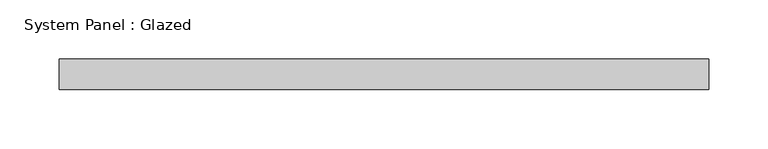
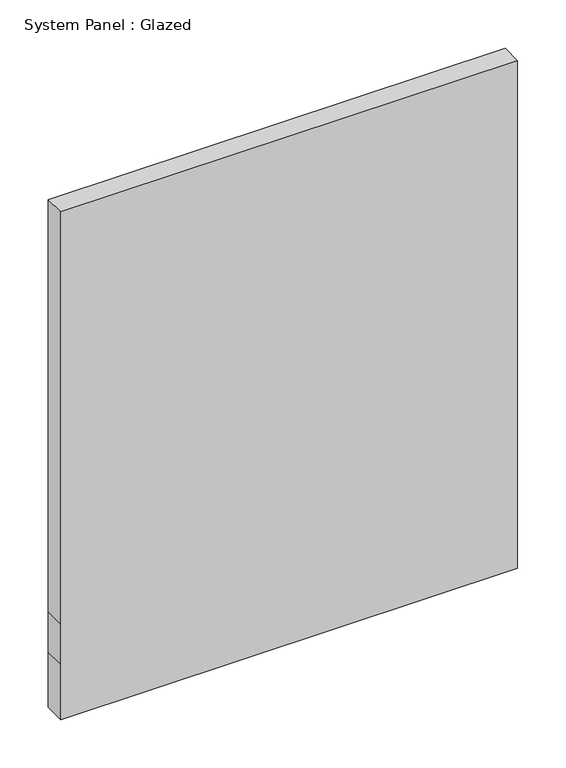
"""IFC4 building model written with IfcOpenShell, lengths in millimetres: plate geometry, System Panel : Glazed."""

from ifc_helpers import new_model, si_unit, frame, origin, place, context, project, spatial, polyline, outline, extrude, source, transform, mapped, element, save


def system_panel_glazed_693ea391(model_context):
    return source(origin(), model_context, "Body", "SweptSolid", [
        extrude(outline(polyline([(0.0, -273.05), (0.0, 273.05), (69.85, 273.05), (120.65, 273.05), (641.0467564, 273.05), (641.0467564, -273.05), (120.65, -273.05), (69.85, -273.05), (0.0, -273.05)])), frame((0.0, 19.05, 0.0), z_axis=(0.0, 1.0, 0.0), x_axis=(0.0, 0.0, 1.0)), (0.0, 0.0, 1.0), 25.4),
    ])


if __name__ == "__main__":
    model = new_model("IFC4")
    model_context = context("Model", 3, world=origin())
    ifc_project = project(units=[si_unit("LENGTHUNIT", "METRE", prefix="MILLI")], contexts=[model_context])
    site = spatial("IfcSite", under=ifc_project)
    building = spatial("IfcBuilding", under=site)
    placement = place(None, origin())
    system_panel_glazed_shape = system_panel_glazed_693ea391(model_context)
    element("IfcPlate", 1, ObjectType="System Panel : Glazed", at=placement, inside=building, context=model_context, shape_type="MappedRepresentation", body=[
        mapped(system_panel_glazed_shape, transform((0.0, 0.0, 0.0), x_axis=(1.0, 0.0, 0.0), y_axis=(0.0, 1.0, 0.0), z_axis=(0.0, 0.0, 1.0))),
    ])
    save(model, "model.ifc")

# Revit data of these elements
# Type "System Panel : Glazed"
#   Construction Type Id = "GSP4R"
#   Analytic Construction = "1/8 in Pilkington single glazing"
#   Visual Light Transmittance = 0.9
#   Solar Heat Gain Coefficient = 0.86
#   Heat Transfer Coefficient (U) = 1.18115 BTU/(h·ft²·°F)
#   Define Thermal Properties by = 1
# Element 1 (IfcPlate, "System Panel : Glazed")
#   Materials on its faces: "Glass"
# Materials
#   "Glass": class "Glass", colour RGB 0 128 192, transparency 0.75, Description = "Soda Lime Glass", Cost = 0
